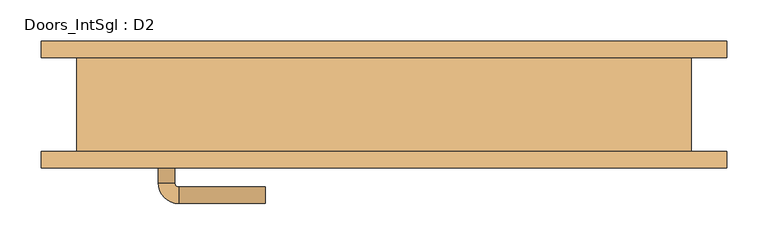
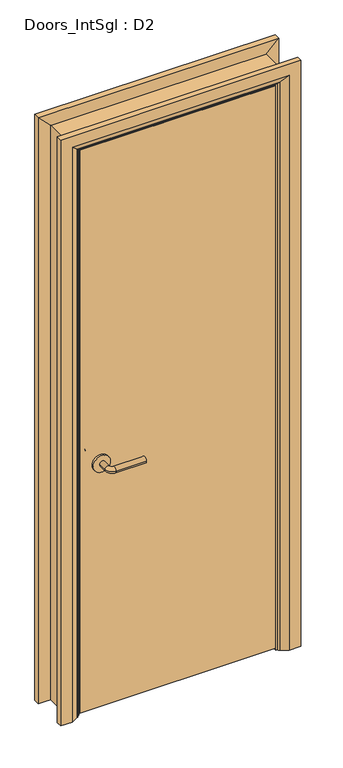
"""IFC4 building model written with IfcOpenShell, lengths in millimetres: door geometry, Doors_IntSgl : D2."""

from ifc_helpers import new_model, si_unit, point, frame, frame_2d, origin, place, context, project, spatial, polyline, circle_curve, ellipse_curve, trimmed, segment, composite_curve, outline, extrude, faceted_brep, source, transform, mapped, element, save
from ifc_brep_helpers import plane_surface, cylinder_surface, revolved_surface, advanced_brep


def doors_intsgl_d2_1f5f3f16(model_context):
    return source(origin(), model_context, "Body", "SolidModel", [
        advanced_brep(
        [(-274.0, -11.15, 900.0), (-254.0, -11.15, 900.0), (-274.0, 18.85, 900.0), (-254.0, 18.85, 900.0), (-249.0, 23.85, 900.0), (-249.0, 43.85, 900.0), (-144.0, 43.85, 900.0), (-144.0, 23.85, 900.0)],
        [
            (0, 1, circle_curve(frame((-264.0, -11.15, 900.0), z_axis=(0.0, -1.0, 0.0), x_axis=(1.0, 0.0, 0.0)), 10.0)),
            (1, 0, circle_curve(frame((-264.0, -11.15, 900.0), z_axis=(0.0, -1.0, 0.0), x_axis=(1.0, 0.0, 0.0)), 10.0)),
            (0, 2),
            (2, 3, circle_curve(frame((-264.0, 18.85, 900.0), z_axis=(0.0, -1.0, 0.0), x_axis=(1.0, 0.0, 0.0)), 10.0)),
            (3, 1),
            (3, 2, circle_curve(frame((-264.0, 18.85, 900.0), z_axis=(0.0, -1.0, 0.0), x_axis=(1.0, 0.0, 0.0)), 10.0)),
            (4, 3, circle_curve(frame((-249.0, 18.85, 900.0), z_axis=(0.0, 0.0, 1.0), x_axis=(-1.0, 0.0, 0.0)), 5.0)),
            (2, 5, circle_curve(frame((-249.0, 18.85, 900.0), z_axis=(0.0, 0.0, -1.0), x_axis=(-1.0, 0.0, 0.0)), 25.0)),
            (5, 4, circle_curve(frame((-249.0, 33.85, 900.0), z_axis=(-1.0, 0.0, 0.0), x_axis=(0.0, -1.0, 0.0)), 10.0)),
            (4, 5, circle_curve(frame((-249.0, 33.85, 900.0), z_axis=(-1.0, 0.0, 0.0), x_axis=(0.0, -1.0, 0.0)), 10.0)),
            (6, 7, circle_curve(frame((-144.0, 33.85, 900.0), z_axis=(1.0, 0.0, 0.0), x_axis=(0.0, -1.0, 0.0)), 10.0)),
            (7, 6, circle_curve(frame((-144.0, 33.85, 900.0), z_axis=(1.0, 0.0, 0.0), x_axis=(0.0, -1.0, 0.0)), 10.0)),
            (5, 6),
            (7, 4),
        ],
        [
            plane_surface(frame((-264.0, -11.15, 900.0), z_axis=(0.0, -1.0, 0.0), x_axis=(0.0, 0.0, 1.0))),
            cylinder_surface(frame((-264.0, -11.15, 900.0), z_axis=(0.0, -1.0, 0.0), x_axis=(1.0, 0.0, 0.0)), 10.0),
            revolved_surface(trimmed(ellipse_curve(frame((-264.0, 18.85, 900.0), z_axis=(0.0, -1.0, 0.0), x_axis=(1.0, 0.0, 0.0)), 10.0, 10.0), [point((-274.0, 18.85, 900.0))], [point((-254.0, 18.85, 900.0))], True, "CARTESIAN"), (-249.0, 18.85, 900.0), (0.0, 0.0, -1.0)),
            revolved_surface(trimmed(ellipse_curve(frame((-264.0, 18.85, 900.0), z_axis=(0.0, -1.0, 0.0), x_axis=(1.0, 0.0, 0.0)), 10.0, 10.0), [point((-254.0, 18.85, 900.0))], [point((-274.0, 18.85, 900.0))], True, "CARTESIAN"), (-249.0, 18.85, 900.0), (0.0, 0.0, -1.0)),
            plane_surface(frame((-144.0, 33.85, 900.0), z_axis=(1.0, 0.0, 0.0), x_axis=(0.0, 0.0, 1.0))),
            cylinder_surface(frame((-249.0, 33.85, 900.0), z_axis=(-1.0, 0.0, 0.0), x_axis=(0.0, -1.0, 0.0)), 10.0),
        ],
        [
            (0, [[1, 2]]),
            (1, [[-1, 3, 4, 5]]),
            (1, [[-2, -5, 6, -3]]),
            (2, [[7, -4, 8, 9]]),
            (3, [[-8, -6, -7, 10]]),
            (4, [[11, 12]]),
            (5, [[-9, 13, -12, 14]]),
            (5, [[-10, -14, -11, -13]]),
        ],
    ),
        extrude(outline(composite_curve([segment(trimmed(circle_curve(frame_2d((900.0, -266.5)), 30.0), [point((900.0, -296.5))], [point((900.0, -236.5))], False, "CARTESIAN"), True, "CONTINUOUS"), segment(trimmed(circle_curve(frame_2d((900.0, -266.5)), 30.0), [point((900.0, -236.5))], [point((900.0, -296.5))], False, "CARTESIAN"), True, "CONTINUOUS")], self_intersect=False)), frame((0.0, -19.15, 0.0), z_axis=(0.0, 1.0, 0.0), x_axis=(0.0, 0.0, 1.0)), (0.0, 0.0, 1.0), 8.0),
        advanced_brep(
        [(-274.0, -65.15, 900.0), (-254.0, -65.15, 900.0), (-254.0, -95.15, 900.0), (-274.0, -95.15, 900.0), (-249.0, -100.15, 900.0), (-249.0, -120.15, 900.0), (-144.0, -120.15, 900.0), (-144.0, -100.15, 900.0)],
        [
            (0, 1, circle_curve(frame((-264.0, -65.15, 900.0), z_axis=(0.0, 1.0, 0.0), x_axis=(1.0, 0.0, 0.0)), 10.0)),
            (1, 0, circle_curve(frame((-264.0, -65.15, 900.0), z_axis=(0.0, 1.0, 0.0), x_axis=(1.0, 0.0, 0.0)), 10.0)),
            (1, 2),
            (2, 3, circle_curve(frame((-264.0, -95.15, 900.0), z_axis=(0.0, 1.0, 0.0), x_axis=(1.0, 0.0, 0.0)), 10.0)),
            (3, 0),
            (3, 2, circle_curve(frame((-264.0, -95.15, 900.0), z_axis=(0.0, 1.0, 0.0), x_axis=(1.0, 0.0, 0.0)), 10.0)),
            (4, 5, circle_curve(frame((-249.0, -110.15, 900.0), z_axis=(-1.0, 0.0, 0.0), x_axis=(0.0, 1.0, 0.0)), 10.0)),
            (5, 3, circle_curve(frame((-249.0, -95.15, 900.0), z_axis=(0.0, 0.0, -1.0), x_axis=(-1.0, 0.0, 0.0)), 25.0)),
            (2, 4, circle_curve(frame((-249.0, -95.15, 900.0), z_axis=(0.0, 0.0, 1.0), x_axis=(-1.0, 0.0, 0.0)), 5.0)),
            (5, 4, circle_curve(frame((-249.0, -110.15, 900.0), z_axis=(-1.0, 0.0, 0.0), x_axis=(0.0, 1.0, 0.0)), 10.0)),
            (6, 7, circle_curve(frame((-144.0, -110.15, 900.0), z_axis=(1.0, 0.0, 0.0), x_axis=(0.0, 1.0, 0.0)), 10.0)),
            (7, 6, circle_curve(frame((-144.0, -110.15, 900.0), z_axis=(1.0, 0.0, 0.0), x_axis=(0.0, 1.0, 0.0)), 10.0)),
            (4, 7),
            (6, 5),
        ],
        [
            plane_surface(frame((-264.0, -65.15, 900.0), z_axis=(0.0, 1.0, 0.0), x_axis=(0.0, 0.0, 1.0))),
            cylinder_surface(frame((-264.0, -65.15, 900.0), z_axis=(0.0, 1.0, 0.0), x_axis=(1.0, 0.0, 0.0)), 10.0),
            revolved_surface(trimmed(ellipse_curve(frame((-264.0, -95.15, 900.0), z_axis=(0.0, -1.0, 0.0), x_axis=(1.0, 0.0, 0.0)), 10.0, 10.0), [point((-274.0, -95.15, 900.0))], [point((-254.0, -95.15, 900.0))], True, "CARTESIAN"), (-249.0, -95.15, 900.0), (0.0, 0.0, -1.0)),
            revolved_surface(trimmed(ellipse_curve(frame((-264.0, -95.15, 900.0), z_axis=(0.0, -1.0, 0.0), x_axis=(1.0, 0.0, 0.0)), 10.0, 10.0), [point((-254.0, -95.15, 900.0))], [point((-274.0, -95.15, 900.0))], True, "CARTESIAN"), (-249.0, -95.15, 900.0), (0.0, 0.0, -1.0)),
            plane_surface(frame((-144.0, -110.15, 900.0), z_axis=(1.0, 0.0, 0.0), x_axis=(0.0, 0.0, 1.0))),
            cylinder_surface(frame((-249.0, -110.15, 900.0), z_axis=(-1.0, 0.0, 0.0), x_axis=(0.0, 1.0, 0.0)), 10.0),
        ],
        [
            (0, [[1, 2]]),
            (1, [[3, 4, 5, -2]]),
            (1, [[-5, 6, -3, -1]]),
            (2, [[7, 8, -4, 9]]),
            (3, [[10, -9, -6, -8]]),
            (4, [[11, 12]]),
            (5, [[13, -11, 14, -7]]),
            (5, [[-14, -12, -13, -10]]),
        ],
    ),
        extrude(outline(composite_curve([segment(trimmed(circle_curve(frame_2d((900.0, -266.5)), 30.0), [point((900.0, -296.5))], [point((900.0, -236.5))], False, "CARTESIAN"), True, "CONTINUOUS"), segment(trimmed(circle_curve(frame_2d((900.0, -266.5)), 30.0), [point((900.0, -236.5))], [point((900.0, -296.5))], False, "CARTESIAN"), True, "CONTINUOUS")], self_intersect=False)), frame((0.0, -65.15, 0.0), z_axis=(0.0, 1.0, 0.0), x_axis=(0.0, 0.0, 1.0)), (0.0, 0.0, 1.0), 8.0),
        extrude(outline(polyline([(339.0, -19.15), (339.0, -57.15), (-339.0, -57.15), (-339.0, -19.15), (339.0, -19.15)])), frame((0.0, 0.0, 8.0), z_axis=(0.0, 0.0, 1.0), x_axis=(1.0, 0.0, 0.0)), (0.0, 0.0, 1.0), 2060.0),
        advanced_brep(
        [(416.0, -77.15, 0.0), (376.0, -77.15, 0.0), (350.0, -63.15, 0.0), (346.0, -57.15, 0.0), (416.0, -57.15, 0.0), (416.0, -57.15, 2145.0), (416.0, -77.15, 2145.0), (346.0, -57.15, 2075.0), (-346.0, -57.15, 2075.0), (-346.0, -57.15, 0.0), (-416.0, -57.15, 0.0), (-416.0, -57.15, 2145.0), (350.0, -63.15, 2079.0), (376.0, -77.15, 2105.0), (-416.0, -77.15, 2145.0), (-416.0, -77.15, 0.0), (-376.0, -77.15, 0.0), (-376.0, -77.15, 2105.0), (-350.0, -63.15, 0.0), (-350.0, -63.15, 2079.0)],
        [
            (0, 1),
            (1, 2),
            (2, 3, circle_curve(frame((354.0, -56.15, 0.0), z_axis=(0.0, 0.0, -1.0), x_axis=(1.0, 0.0, 0.0)), 8.0622577)),
            (3, 4),
            (4, 0),
            (4, 5),
            (5, 6),
            (6, 0),
            (3, 7),
            (7, 8),
            (8, 9),
            (9, 10),
            (10, 11),
            (11, 5),
            (2, 12),
            (12, 7, ellipse_curve(frame((354.0, -56.15, 2083.0), z_axis=(0.7071067811865475, 0.0, -0.7071067811865475), x_axis=(-0.7071067811865474, 0.0, -0.7071067811865476)), 11.4017543, 8.0622577)),
            (1, 13),
            (13, 12),
            (6, 14),
            (14, 15),
            (15, 16),
            (16, 17),
            (17, 13),
            (10, 15),
            (14, 11),
            (9, 18, circle_curve(frame((-354.0, -56.15, 0.0), z_axis=(0.0, 0.0, -1.0), x_axis=(-1.0, 0.0, 0.0)), 8.0622577)),
            (18, 16),
            (19, 18),
            (8, 19, ellipse_curve(frame((-354.0, -56.15, 2083.0), z_axis=(-0.7071067811865475, 0.0, -0.7071067811865475), x_axis=(-0.7071067811865474, 0.0, 0.7071067811865476)), 11.4017543, 8.0622577)),
            (19, 17),
            (12, 19),
        ],
        [
            plane_surface(frame((346.0, -57.15, 0.0), z_axis=(0.0, 0.0, -1.0), x_axis=(0.0, 1.0, 0.0))),
            plane_surface(frame((416.0, -77.15, 0.0), z_axis=(1.0, 0.0, 0.0), x_axis=(0.0, 0.0, 1.0))),
            plane_surface(frame((416.0, -57.15, 0.0), z_axis=(0.0, 1.0, 0.0), x_axis=(0.0, 0.0, 1.0))),
            cylinder_surface(frame((354.0, -56.15, 0.0), z_axis=(0.0, 0.0, -1.0), x_axis=(1.0, 0.0, 0.0)), 8.0622577),
            plane_surface(frame((350.0, -63.15, 0.0), z_axis=(-0.4740998230350126, -0.880471099922178, 0.0), x_axis=(0.0, 0.0, 1.0))),
            plane_surface(frame((376.0, -77.15, 0.0), z_axis=(0.0, -1.0, 0.0), x_axis=(0.0, 0.0, 1.0))),
            plane_surface(frame((-416.0, -77.15, 2145.0), z_axis=(-1.0, 0.0, 0.0), x_axis=(0.0, 0.0, -1.0))),
            plane_surface(frame((-346.0, -57.15, 0.0), z_axis=(0.0, 0.0, -1.0), x_axis=(0.0, 1.0, 0.0))),
            cylinder_surface(frame((-354.0, -56.15, 2075.0), z_axis=(0.0, 0.0, 1.0), x_axis=(-1.0, 0.0, 0.0)), 8.0622577),
            plane_surface(frame((-350.0, -63.15, 2079.0), z_axis=(0.47409982303501824, -0.8804710999221749, 0.0), x_axis=(0.0, 0.0, -1.0))),
            plane_surface(frame((416.0, -77.15, 2145.0), z_axis=(0.0, 0.0, 1.0), x_axis=(-1.0, 0.0, 0.0))),
            cylinder_surface(frame((346.0, -56.15, 2083.0), z_axis=(1.0, 0.0, 0.0), x_axis=(0.0, 0.0, 1.0)), 8.0622577),
            plane_surface(frame((350.0, -63.15, 2079.0), z_axis=(0.0, -0.8804710999221764, -0.4740998230350154), x_axis=(-1.0, 0.0, 0.0))),
        ],
        [
            (0, [[1, 2, 3, 4, 5]]),
            (1, [[6, 7, 8, -5]]),
            (2, [[9, 10, 11, 12, 13, 14, -6, -4]]),
            (3, [[15, 16, -9, -3]]),
            (4, [[17, 18, -15, -2]]),
            (5, [[-8, 19, 20, 21, 22, 23, -17, -1]]),
            (6, [[-13, 24, -20, 25]]),
            (7, [[-24, -12, 26, 27, -21]]),
            (8, [[28, -26, -11, 29]]),
            (9, [[-22, -27, -28, 30]]),
            (10, [[-14, -25, -19, -7]]),
            (11, [[31, -29, -10, -16]]),
            (12, [[-23, -30, -31, -18]]),
        ],
    ),
        extrude(outline(polyline([(0.0, -322.0), (2051.0, -322.0), (2051.0, 322.0), (0.0, 322.0), (0.0, 341.0), (2070.0, 341.0), (2070.0, -341.0), (0.0, -341.0), (0.0, -322.0)])), frame((0.0, -17.15, 0.0), z_axis=(0.0, 1.0, 0.0), x_axis=(0.0, 0.0, 1.0)), (0.0, 0.0, 1.0), 32.0),
        advanced_brep(
        [(-416.0, 77.15, 0.0), (-376.0, 77.15, 0.0), (-350.0, 63.15, 0.0), (-346.0, 57.15, 0.0), (-416.0, 57.15, 0.0), (-416.0, 57.15, 2145.0), (-416.0, 77.15, 2145.0), (-346.0, 57.15, 2075.0), (-350.0, 63.15, 2079.0), (-376.0, 77.15, 2105.0), (416.0, 77.15, 0.0), (416.0, 57.15, 0.0), (346.0, 57.15, 0.0), (350.0, 63.15, 0.0), (376.0, 77.15, 0.0), (416.0, 77.15, 2145.0), (376.0, 77.15, 2105.0), (350.0, 63.15, 2079.0), (346.0, 57.15, 2075.0), (416.0, 57.15, 2145.0)],
        [
            (0, 1),
            (1, 2),
            (2, 3, circle_curve(frame((-354.0, 56.15, 0.0), z_axis=(0.0, 0.0, -1.0), x_axis=(-1.0, 0.0, 0.0)), 8.0622577)),
            (3, 4),
            (4, 0),
            (4, 5),
            (5, 6),
            (6, 0),
            (3, 7),
            (7, 5),
            (2, 8),
            (8, 7, ellipse_curve(frame((-354.0, 56.15, 2083.0), z_axis=(-0.7071067811865475, 0.0, -0.7071067811865475), x_axis=(0.7071067811865474, 0.0, -0.7071067811865476)), 11.4017543, 8.0622577)),
            (1, 9),
            (9, 8),
            (6, 9),
            (10, 11),
            (11, 12),
            (12, 13, circle_curve(frame((354.0, 56.15, 0.0), z_axis=(0.0, 0.0, -1.0), x_axis=(1.0, 0.0, 0.0)), 8.0622577)),
            (13, 14),
            (14, 10),
            (15, 10),
            (14, 16),
            (16, 15),
            (13, 17),
            (17, 16),
            (12, 18),
            (18, 17, ellipse_curve(frame((354.0, 56.15, 2083.0), z_axis=(0.7071067811865475, 0.0, -0.7071067811865475), x_axis=(0.7071067811865474, 0.0, 0.7071067811865476)), 11.4017543, 8.0622577)),
            (11, 19),
            (19, 18),
            (15, 19),
            (5, 19),
            (15, 6),
            (7, 18),
            (8, 17),
            (9, 16),
        ],
        [
            plane_surface(frame((-346.0, 129.9510989, 0.0), z_axis=(0.0, 0.0, -1.0), x_axis=(1.0, 0.0, 0.0))),
            plane_surface(frame((-416.0, 77.15, 0.0), z_axis=(-1.0, 0.0, 0.0), x_axis=(0.0, 0.0, 1.0))),
            plane_surface(frame((-416.0, 57.15, 0.0), z_axis=(0.0, -1.0, 0.0), x_axis=(0.0, 0.0, 1.0))),
            cylinder_surface(frame((-354.0, 56.15, 0.0), z_axis=(0.0, 0.0, -1.0), x_axis=(-1.0, 0.0, 0.0)), 8.0622577),
            plane_surface(frame((-350.0, 63.15, 0.0), z_axis=(0.4740998230350183, 0.8804710999221749, 0.0), x_axis=(0.0, 0.0, 1.0))),
            plane_surface(frame((-376.0, 77.15, 0.0), z_axis=(0.0, 1.0, 0.0), x_axis=(0.0, 0.0, 1.0))),
            plane_surface(frame((346.0, 129.9510989, 0.0), z_axis=(0.0, 0.0, -1.0), x_axis=(-1.0, 0.0, 0.0))),
            plane_surface(frame((376.0, 77.15, 2105.0), z_axis=(0.0, 1.0, 0.0), x_axis=(0.0, 0.0, -1.0))),
            plane_surface(frame((350.0, 63.15, 2079.0), z_axis=(-0.4740998230350183, 0.8804710999221749, 0.0), x_axis=(0.0, 0.0, -1.0))),
            cylinder_surface(frame((354.0, 56.15, 2075.0), z_axis=(0.0, 0.0, 1.0), x_axis=(1.0, 0.0, 0.0)), 8.0622577),
            plane_surface(frame((416.0, 57.15, 2145.0), z_axis=(0.0, -1.0, 0.0), x_axis=(0.0, 0.0, -1.0))),
            plane_surface(frame((416.0, 77.15, 2145.0), z_axis=(1.0, 0.0, 0.0), x_axis=(0.0, 0.0, -1.0))),
            plane_surface(frame((-416.0, 77.15, 2145.0), z_axis=(0.0, 0.0, 1.0), x_axis=(1.0, 0.0, 0.0))),
            plane_surface(frame((-416.0, 57.15, 2145.0), z_axis=(0.0, -1.0, 0.0), x_axis=(1.0, 0.0, 0.0))),
            cylinder_surface(frame((-346.0, 56.15, 2083.0), z_axis=(-1.0, 0.0, 0.0), x_axis=(0.0, 0.0, 1.0)), 8.0622577),
            plane_surface(frame((-350.0, 63.15, 2079.0), z_axis=(0.0, 0.8804710999221749, -0.4740998230350183), x_axis=(1.0, 0.0, 0.0))),
            plane_surface(frame((-376.0, 77.15, 2105.0), z_axis=(0.0, 1.0, 0.0), x_axis=(1.0, 0.0, 0.0))),
        ],
        [
            (0, [[1, 2, 3, 4, 5]]),
            (1, [[6, 7, 8, -5]]),
            (2, [[9, 10, -6, -4]]),
            (3, [[11, 12, -9, -3]]),
            (4, [[13, 14, -11, -2]]),
            (5, [[-8, 15, -13, -1]]),
            (6, [[16, 17, 18, 19, 20]]),
            (7, [[21, -20, 22, 23]]),
            (8, [[-22, -19, 24, 25]]),
            (9, [[-24, -18, 26, 27]]),
            (10, [[-26, -17, 28, 29]]),
            (11, [[-28, -16, -21, 30]]),
            (12, [[31, -30, 32, -7]]),
            (13, [[33, -29, -31, -10]]),
            (14, [[34, -27, -33, -12]]),
            (15, [[35, -25, -34, -14]]),
            (16, [[-32, -23, -35, -15]]),
        ],
    ),
        faceted_brep([(-341.0, -57.15, 0.0), (-373.0, -57.15, 0.0), (-373.0, 57.15, 0.0), (-341.0, 57.15, 0.0), (-341.0, 57.15, 2070.0), (-341.0, -57.15, 2070.0), (-373.0, 57.15, 2102.0), (-373.0, -57.15, 2102.0), (341.0, -57.15, 0.0), (341.0, 57.15, 0.0), (373.0, 57.15, 0.0), (373.0, -57.15, 0.0), (341.0, -57.15, 2070.0), (373.0, -57.15, 2102.0), (373.0, 57.15, 2102.0), (341.0, 57.15, 2070.0)], [[[0, 1, 2, 3]], [[3, 4, 5, 0]], [[2, 6, 4, 3]], [[1, 7, 6, 2]], [[0, 5, 7, 1]], [[8, 9, 10, 11]], [[12, 8, 11, 13]], [[13, 11, 10, 14]], [[14, 10, 9, 15]], [[15, 9, 8, 12]], [[4, 15, 12, 5]], [[6, 14, 15, 4]], [[7, 13, 14, 6]], [[5, 12, 13, 7]]]),
    ])


if __name__ == "__main__":
    model = new_model("IFC4")
    model_context = context("Model", 3, world=origin())
    ifc_project = project(units=[si_unit("LENGTHUNIT", "METRE", prefix="MILLI")], contexts=[model_context])
    site = spatial("IfcSite", under=ifc_project)
    building = spatial("IfcBuilding", under=site)
    placement = place(None, origin())
    doors_intsgl_d2_shape = doors_intsgl_d2_1f5f3f16(model_context)
    element("IfcDoor", 1, ObjectType="Doors_IntSgl : D2", at=placement, inside=building, context=model_context, shape_type="MappedRepresentation", body=[
        mapped(doors_intsgl_d2_shape, transform((0.0, 0.0, 0.0), x_axis=(1.0, 0.0, 0.0), y_axis=(0.0, 1.0, 0.0), z_axis=(0.0, 0.0, 1.0))),
    ])
    save(model, "model.ifc")

# Revit data of these elements
# Type "Doors_IntSgl : D2"
#   Type Mark = "47"
#   Type Comments = "Internal Single"
#   Operation = "SingleSwingRight"
#   Manufacturer = "Revit"
#   Keynote = "L20"
#   Description = "Internal Single Door"
#   Analytic Construction = "Metal"
#   UnderCut = 0.026247 ft
#   Tolerance = 0.006562 ft
#   Thickness = 0.124672 ft
#   Thermal Resistance (R) = 0.270117 (m²·K)/W
#   Structural Tolerance = 0.026247 ft
#   StopDepth = 0.104987 ft
#   Stop Thickness = 0.062336 ft
#   Rough Width = 2.5 ft
#   Rough Height = 6.922572 ft
#   Height to Top Lock Rail = 3.28084 ft
#   Heat Transfer Coefficient (U) = 3.7021 W/(m²·K)
#   Handle Z Distance = 2.952756 ft
#   Handle X Distance = 0.246063 ft
#   Frame Thickness = 0.104987 ft
#   Door Panel Width = 2.224409 ft
#   Door Panel Thickness = 0.124672 ft
#   Door Panel Offset = 0.0 ft
#   Height = 6.922572 ft
#   Width = 2.5 ft
#   Door Panel Height = 6.75853 ft
#   Architrave Setback = 0.016404 ft
#   Vis - Ironmongery = yes
#   Material Ironmongery = Door - Handle
#   Material Frame = Door - Frame/Mullion (1)
#   Material Door = Door - Panel
#   Material Architrave = Door - Architrave
#   Visual Light Transmittance = 0
#   Solar Heat Gain Coefficient = 0
#   Function = (empty or 0)
#   Wall Closure = (empty or 0)
# Element 1 (IfcDoor, "Doors_IntSgl : D2")
#   Materials on its faces: "Door - Architrave", "Door - Handle", "Door - Frame/Mullion (1)", "Door - Panel"
# Materials
#   "Door - Handle": colour RGB 0 0 0, transparency 0, Keynote = "P21", Cost = 0
#   "Door - Frame/Mullion (1)": class "Wood", colour RGB 212 179 113, transparency 0, Keynote = "L20", Cost = 0
#   "Door - Panel": class "Wood", colour RGB 210 159 95, transparency 0, Keynote = "L20", Cost = 0
#   "Door - Architrave": class "Wood", colour RGB 154 90 5, transparency 0, Keynote = "P20", Cost = 0
